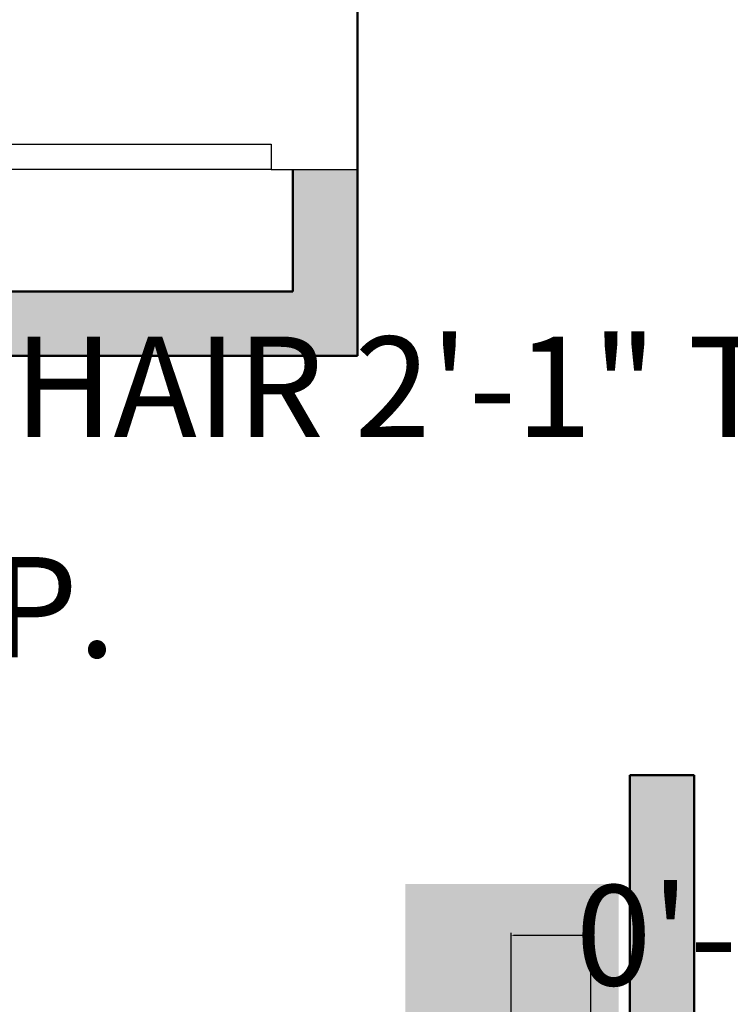
# Model space of a CAD drawing. Units: inches. Extents: x 2974 to 3443, y 2405 to 2963.
# Tile 4 of 13: x 3165 to 3214, y 2642 to 2711. Entities that reach past the tile are written whole.
import ezdxf

# ---------------------------------------------------------------- set-up
doc = ezdxf.new("R2010")
doc.units = ezdxf.units.IN
doc.header["$MEASUREMENT"] = 0
doc.layers.get('0').update_dxf_attribs({"color": 251})
for name, color, linetype, lineweight in [('A-ANNO-DIMS', 2, 'Continuous', 18), ('A-DOOR', 32, 'Continuous', 25), ('A-WALL-PATT', 252, 'Continuous', 13), ('walls', 250, 'Continuous', 50)]:
    doc.layers.add(name, color=color, linetype=linetype, lineweight=lineweight)
doc.layers.add('A-FURN-PATT', color=254, linetype='Continuous', lineweight=13, true_color=0xfeeab9)
doc.styles.get("Standard").update_dxf_attribs({"font": 'arial.ttf'})
doc.dimstyles.get("Standard").update_dxf_attribs({"dimtxt": 7, "dimasz": 0.18, "dimexe": 0.18, "dimexo": 0.0625, "dimgap": 0.09, "dimtad": 0, "dimtih": 1, "dimtoh": 1, "dimzin": 0, "dimdsep": 46, "dimlunit": 3, "dimtxsty": 'Standard', "dimcen": 0.09, "dimadec": 0, "dimazin": 0, "dimtfac": 1, "dimtofl": 0, "dimtmove": 0, "dimatfit": 3, "dimfxl": 1, "dimtolj": 1, "dimtzin": 0, "dimarcsym": 0})

# ---------------------------------------------------------------- blocks, each defined once
blk = doc.blocks.new('*U2')
for p, q in [((0, 0), (0, -6)), ((40, 0), (40, -6))]:
    blk.add_line(p, q)
blk.add_lwpolyline([(0, 0), (0, 40), (1.75, 40), (1.75, 0)], close=True)
blk.add_arc((0, 0), 40, 0, 90)
blk = doc.blocks.new('*D35')
at = {"layer": 'A-ANNO-DIMS', "color": 0, "lineweight": -2, "transparency": 16777216}
for p, q in [((3110.658, 2681.378), (3110.658, 2685.223)), ((3135.509, 2681.378), (3135.509, 2685.223)), ((3110.838, 2685.043), (3135.329, 2685.043)), ((3135.509, 2685.043), (3135.689, 2685.043))]:
    blk.add_line(p, q, dxfattribs=at)
at = {"layer": 'A-ANNO-DIMS', "color": 0, "transparency": 16777216}
for points in [[(3110.838, 2685.073), (3110.838, 2685.013), (3110.658, 2685.043)], [(3135.329, 2685.073), (3135.329, 2685.013), (3135.509, 2685.043)]]:
    blk.add_solid(points, dxfattribs=at)
at = {"layer": 'Defpoints', "color": 0, "transparency": 16777216}
for p in [(3135.509, 2685.043), (3110.658, 2681.315), (3135.509, 2681.315)]:
    blk.add_point(p, dxfattribs=at)
at = {"layer": 'A-ANNO-DIMS', "color": 0, "transparency": 16777216, "insert": (3184.753, 2685.043), "char_height": 7, "attachment_point": 5}
blk.add_mtext('\\A1;ARMCHAIR 2\'-1" TYP.', dxfattribs=at)
blk = doc.blocks.new('*D36')
at = {"layer": 'A-ANNO-DIMS', "color": 0, "lineweight": -2, "transparency": 16777216}
for p, q in [((3135.571, 2681.315), (3139.417, 2681.315)), ((3139.237, 2681.135), (3139.237, 2673.371)), ((3139.237, 2658.187), (3139.237, 2665.952)), ((3135.571, 2658.007), (3139.417, 2658.007))]:
    blk.add_line(p, q, dxfattribs=at)
at = {"layer": 'A-ANNO-DIMS', "color": 0, "transparency": 16777216}
for points in [[(3139.207, 2681.135), (3139.267, 2681.135), (3139.237, 2681.315)], [(3139.207, 2658.187), (3139.267, 2658.187), (3139.237, 2658.007)]]:
    blk.add_solid(points, dxfattribs=at)
at = {"layer": 'Defpoints', "color": 0, "transparency": 16777216}
for p in [(3135.509, 2681.315), (3135.509, 2658.007), (3139.237, 2658.007)]:
    blk.add_point(p, dxfattribs=at)
at = {"layer": 'A-ANNO-DIMS', "color": 0, "transparency": 16777216, "insert": (3139.237, 2669.661), "char_height": 7, "attachment_point": 5}
blk.add_mtext('\\A1;1\'-11 1/2" TYP.', dxfattribs=at)
blk = doc.blocks.new('*D46')
at = {"layer": 'A-ANNO-DIMS', "color": 0, "lineweight": -2, "transparency": 16777216}
for p, q in [((3199.048, 2640.453), (3199.048, 2646.942)), ((3199.228, 2646.762), (3204.43, 2646.762)), ((3204.61, 2640.453), (3204.61, 2646.942)), ((3204.61, 2646.762), (3204.79, 2646.762))]:
    blk.add_line(p, q, dxfattribs=at)
at = {"layer": 'A-ANNO-DIMS', "color": 0, "transparency": 16777216}
for points in [[(3199.228, 2646.792), (3199.228, 2646.732), (3199.048, 2646.762)], [(3204.43, 2646.792), (3204.43, 2646.732), (3204.61, 2646.762)]]:
    blk.add_solid(points, dxfattribs=at)
at = {"layer": 'Defpoints', "color": 0, "transparency": 16777216}
for p in [(3204.61, 2646.762), (3199.048, 2640.391), (3204.61, 2640.391)]:
    blk.add_point(p, dxfattribs=at)
at = {"layer": 'A-ANNO-DIMS', "color": 0, "transparency": 16777216, "insert": (3222.339, 2646.762), "char_height": 7, "attachment_point": 5}
blk.add_mtext('\\A1;0\'-5 1/2"', dxfattribs=at)
blk = doc.blocks.new('*D47')
at = {"layer": 'A-ANNO-DIMS', "color": 0, "lineweight": -2, "transparency": 16777216}
for p, q in [((3247.425, 2644.017), (3247.425, 2630.764)), ((3334.991, 2644.017), (3334.991, 2630.764)), ((3247.425, 2630.944), (3247.245, 2630.944)), ((3334.811, 2630.944), (3247.605, 2630.944))]:
    blk.add_line(p, q, dxfattribs=at)
at = {"layer": 'A-ANNO-DIMS', "color": 0, "transparency": 16777216}
for points in [[(3247.605, 2630.974), (3247.605, 2630.914), (3247.425, 2630.944)], [(3334.811, 2630.974), (3334.811, 2630.914), (3334.991, 2630.944)]]:
    blk.add_solid(points, dxfattribs=at)
at = {"layer": 'Defpoints', "color": 0, "transparency": 16777216}
for p in [(3247.425, 2644.079), (3334.991, 2644.079), (3247.425, 2630.944)]:
    blk.add_point(p, dxfattribs=at)
at = {"layer": 'A-ANNO-DIMS', "color": 0, "transparency": 16777216, "insert": (3200.531, 2630.944), "char_height": 7, "attachment_point": 5}
blk.add_mtext('\\A1;DINING SET 7\'-3 1/2"', dxfattribs=at)

msp = doc.modelspace()

# ---------------------------------------------------------------- hatches: boundary and pattern name
at = {"layer": 'A-FURN-PATT'}
h = msp.add_hatch(color=256, dxfattribs=at)
h.dxf.hatch_style = 1
h.paths.add_polyline_path([(3191.663, 2650.336), (3206.56, 2650.336), (3206.56, 2585.893), (3191.663, 2585.893)])
h.paths.add_polyline_path([(3201.071, 2597.916), (3202.082, 2597.916, 0.064042), (3203.599, 2600.336), (3203.599, 2611.063), (3203.857, 2611.063, 0.414214), (3204.61, 2611.816), (3204.61, 2626.491, 0.414214), (3203.857, 2627.244), (3203.599, 2627.244), (3203.599, 2637.972, 0.064042), (3202.082, 2640.391), (3201.071, 2640.391), (3201.071, 2627.244), (3199.801, 2627.244, 0.414214), (3199.048, 2626.491), (3199.048, 2611.816, 0.414214), (3199.801, 2611.063), (3201.071, 2611.063)], flags=16)
at = {"layer": 'A-WALL-PATT'}
h = msp.add_hatch(color=256, dxfattribs=at)
h.dxf.hatch_style = 1
h.paths.add_polyline_path([(3222.294, 2555.188), (3211.826, 2555.188), (3211.826, 2657.938), (3207.326, 2657.938), (3207.326, 2555.188), (3051.326, 2555.188), (3051.326, 2583.943), (3042.326, 2583.943), (3042.326, 2471.188), (3165.027, 2471.188), (3165.027, 2480.188), (3051.326, 2480.188), (3051.326, 2550.688), (3222.294, 2550.688)])
h.paths.add_polyline_path([(3188.326, 2700.207), (3183.826, 2700.207), (3183.826, 2691.688), (3051.326, 2691.688), (3051.326, 2740.572), (3042.326, 2740.572), (3042.326, 2651.235), (3045.517, 2651.235), (3051.326, 2651.235), (3051.326, 2687.188), (3188.326, 2687.188)])
h.paths.add_polyline_path([(3051.326, 2894.188), (3074.298, 2894.188), (3074.298, 2903.188), (3042.326, 2903.188), (3042.326, 2807.864), (3045.517, 2807.864), (3051.326, 2807.864), (3051.326, 2835.688), (3103.457, 2835.688), (3103.457, 2839.066, -0.012473), (3103.485, 2840.188), (3051.326, 2840.188)])
h.paths.add_polyline_path([(3201.987, 2903.188), (3100.263, 2903.188), (3100.263, 2894.188), (3131.326, 2894.188), (3131.326, 2835.688), (3135.826, 2835.688), (3135.826, 2894.188), (3183.826, 2894.188), (3183.826, 2840.188), (3159.826, 2840.188), (3159.826, 2835.688), (3183.826, 2835.688), (3183.826, 2740.207), (3188.326, 2740.207), (3188.326, 2803.688), (3215.422, 2803.688), (3215.422, 2807.066, -0.012473), (3215.45, 2808.188), (3188.326, 2808.188), (3188.326, 2894.188), (3201.987, 2894.188)])
h.paths.add_polyline_path([(3283.564, 2903.188), (3227.952, 2903.188), (3227.952, 2894.188), (3240.326, 2894.188), (3240.326, 2755.688), (3188.326, 2755.688), (3188.326, 2751.188), (3244.826, 2751.188), (3244.826, 2757.188), (3244.826, 2797.188), (3244.826, 2894.188), (3283.564, 2894.188)])
h.paths.add_polyline_path([(3384.326, 2903.188), (3346.694, 2903.188), (3346.694, 2894.188), (3375.326, 2894.188), (3375.326, 2755.688), (3284.826, 2755.688), (3284.826, 2751.188), (3375.326, 2751.188), (3375.326, 2710.653), (3378.517, 2710.653), (3384.326, 2710.653)])
h.paths.add_polyline_path([(3384.326, 2643.361), (3375.326, 2643.361), (3375.326, 2609.188), (3330.003, 2609.188), (3330.003, 2604.688), (3375.326, 2604.688), (3375.326, 2480.188), (3356.49, 2480.188), (3356.49, 2471.188), (3384.326, 2471.188)])
h.paths.add_polyline_path([(3267.326, 2609.188), (3262.826, 2609.188), (3262.826, 2555.188), (3257.429, 2555.188), (3257.429, 2550.688), (3262.826, 2550.688), (3262.826, 2471.188), (3293.36, 2471.188), (3293.36, 2480.188), (3267.326, 2480.188)])
h.paths.add_polyline_path([(3275.186, 2471.188), (3268.471, 2471.188), (3268.471, 2455.229), (3268.471, 2452.413), (3275.186, 2452.413)])
h.paths.add_polyline_path([(3156.684, 2471.188), (3149.969, 2471.188), (3149.969, 2452.413), (3156.684, 2452.413)])

# ---------------------------------------------------------------- linework, layer by layer
at = {"layer": 'walls'}
for p, q in [((3188.326, 2687.188), (3188.326, 2803.688)), ((3183.826, 2691.688), (3183.826, 2700.207)), ((3051.326, 2691.688), (3183.826, 2691.688)), ((3051.326, 2687.188), (3188.326, 2687.188)), ((3207.326, 2555.188), (3207.326, 2657.938)), ((3211.826, 2657.938), (3207.326, 2657.938)), ((3211.826, 2555.188), (3211.826, 2657.938))]:
    msp.add_line(p, q, dxfattribs=at)

# ---------------------------------------------------------------- block references
at = {"layer": 'A-DOOR', "rotation": 90}
msp.add_blockref('*U2', (3182.326, 2700.207), dxfattribs=at)

# ---------------------------------------------------------------- dimensions: what is measured, and where the dimension line sits
at = {"layer": 'A-ANNO-DIMS'}
dim = msp.add_linear_dim(base=(3135.509, 2685.043), p1=(3110.658, 2681.315), p2=(3135.509, 2681.315), text='ARMCHAIR <> TYP.', dimstyle='Standard', override={"dimdec": 1, "dimlfac": 1, "dimrnd": 0, "dimzin": 1, "dimdsep": 46, "dimlunit": 4, "dimfrac": 2}, dxfattribs=at)
dim.commit()
dim.dimension.update_dxf_attribs({"geometry": '*D35', "text_midpoint": (3184.753, 2685.043)})
for base, p1, p2, angle, text, picture, middle in [((3139.237, 2658.007), (3135.509, 2681.315), (3135.509, 2658.007), 270, '<> TYP.', '*D36', (3139.237, 2669.661)), ((3247.425, 2630.944), (3334.991, 2644.079), (3247.425, 2644.079), 180, 'DINING SET <>', '*D47', (3200.531, 2630.944))]:
    dim = msp.add_linear_dim(base=base, p1=p1, p2=p2, angle=angle, text=text, dimstyle='Standard', override={"dimdec": 1, "dimlfac": 1, "dimrnd": 0, "dimzin": 1, "dimdsep": 46, "dimlunit": 4, "dimfrac": 2}, dxfattribs=at)
    dim.commit()
    dim.dimension.update_dxf_attribs({"geometry": picture, "text_midpoint": middle})
dim = msp.add_linear_dim(base=(3204.61, 2646.762), p1=(3199.048, 2640.391), p2=(3204.61, 2640.391), dimstyle='Standard', override={"dimdec": 1, "dimlfac": 1, "dimrnd": 0, "dimzin": 1, "dimdsep": 46, "dimlunit": 4, "dimfrac": 2}, dxfattribs=at)
dim.commit()
dim.dimension.update_dxf_attribs({"geometry": '*D46', "text_midpoint": (3222.339, 2646.762)})

doc.saveas('drawing.dxf')
